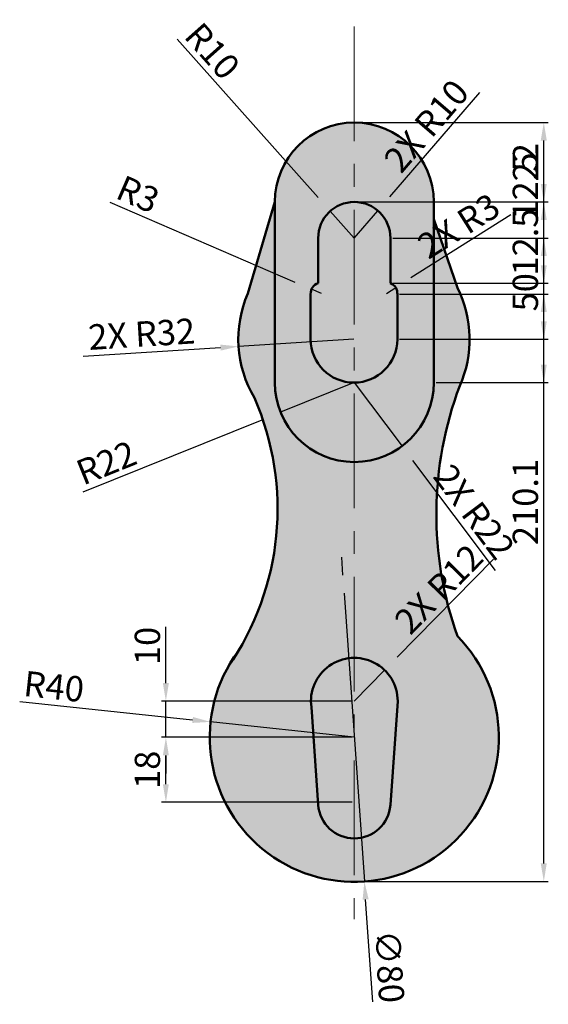
# Model space of a CAD drawing. Units: millimetres. Extents: x 3154 to 3300, y 2281 to 2553.
import ezdxf

# ---------------------------------------------------------------- set-up
doc = ezdxf.new("R2010")
doc.units = ezdxf.units.MM
doc.linetypes.add('CENTER', pattern=[50.8, 31.75, -6.35, 6.35, -6.35])
for name, color, linetype, lineweight in [('M-CNTR', 6, 'CENTER', 18), ('M-CONS', 8, 'Continuous', 13), ('M-DIMS', 2, 'Continuous', 25), ('M-HATC', 252, 'Continuous', 18), ('M-OUTL', 7, 'Continuous', 50)]:
    doc.layers.add(name, color=color, linetype=linetype, lineweight=lineweight)
doc.styles.get("Standard").update_dxf_attribs({"font": 'arial.ttf'})
doc.dimstyles.new('ISO-25', dxfattribs={"dimtxt": 7, "dimasz": 5, "dimexe": 1.25, "dimexo": 0.625, "dimtad": 1, "dimtxsty": 'Standard', "dimcen": 2.5, "dimadec": 0, "dimazin": 0, "dimtfac": 1, "dimtmove": 0, "dimatfit": 3, "dimfxl": 1, "dimarcsym": 0})

# ---------------------------------------------------------------- blocks, each defined once
blk = doc.blocks.new('*D1')
at = {"layer": 'Defpoints', "color": 0, "transparency": 16777216}
for p in [(3239.75, 2500.3), (3246.4, 2492.83)]:
    blk.add_point(p, dxfattribs=at)
at = {"layer": 'M-DIMS', "color": 0, "lineweight": -2, "transparency": 16777216}
for p, q in [((3197.36, 2547.92), (3236.43, 2504.03)), ((3246.4, 2492.83), (3239.75, 2500.3))]:
    blk.add_line(p, q, dxfattribs=at)
at = {"layer": 'M-DIMS', "color": 0, "transparency": 16777216}
blk.add_solid([(3237.05, 2504.59), (3235.8, 2503.48), (3239.75, 2500.3)], dxfattribs=at)
at = {"layer": 'M-DIMS', "color": 0, "transparency": 16777216, "insert": (3206.46, 2544.01), "char_height": 7, "attachment_point": 5, "rotation": 311.6742}
blk.add_mtext('R10', dxfattribs=at)
blk = doc.blocks.new('*D2')
at = {"layer": 'Defpoints', "color": 0, "transparency": 16777216}
for p in [(3246.4, 2452.83), (3225.99, 2444.61)]:
    blk.add_point(p, dxfattribs=at)
at = {"layer": 'M-DIMS', "color": 0, "lineweight": -2, "transparency": 16777216}
for p, q in [((3246.4, 2452.83), (3225.99, 2444.61)), ((3171.35, 2422.6), (3221.35, 2442.74))]:
    blk.add_line(p, q, dxfattribs=at)
at = {"layer": 'M-DIMS', "color": 0, "transparency": 16777216}
blk.add_solid([(3221.04, 2443.52), (3221.67, 2441.97), (3225.99, 2444.61)], dxfattribs=at)
at = {"layer": 'M-DIMS', "color": 0, "transparency": 16777216, "insert": (3178.11, 2429.79), "char_height": 7, "attachment_point": 5, "rotation": 21.936}
blk.add_mtext('R22', dxfattribs=at)
blk = doc.blocks.new('*D3')
at = {"layer": 'Defpoints', "color": 0, "transparency": 16777216}
for p in [(3234.55, 2478.66), (3237.3, 2477.47)]:
    blk.add_point(p, dxfattribs=at)
at = {"layer": 'M-DIMS', "color": 0, "lineweight": -2, "transparency": 16777216}
for p, q in [((3178.78, 2502.78), (3229.96, 2480.64)), ((3237.3, 2477.47), (3234.55, 2478.66))]:
    blk.add_line(p, q, dxfattribs=at)
at = {"layer": 'M-DIMS', "color": 0, "transparency": 16777216}
blk.add_solid([(3230.29, 2481.41), (3229.63, 2479.88), (3234.55, 2478.66)], dxfattribs=at)
at = {"layer": 'M-DIMS', "color": 0, "transparency": 16777216, "insert": (3186.2, 2504.15), "char_height": 7, "attachment_point": 5, "rotation": 336.611}
blk.add_mtext('R3', dxfattribs=at)
blk = doc.blocks.new('*D4')
at = {"layer": 'Defpoints', "color": 0, "transparency": 16777216}
for p in [(3206.63, 2358.9), (3246.4, 2354.63)]:
    blk.add_point(p, dxfattribs=at)
at = {"layer": 'M-DIMS', "color": 0, "lineweight": -2, "transparency": 16777216}
for p, q in [((3153.82, 2364.58), (3201.66, 2359.44)), ((3246.4, 2354.63), (3206.63, 2358.9))]:
    blk.add_line(p, q, dxfattribs=at)
at = {"layer": 'M-DIMS', "color": 0, "transparency": 16777216}
blk.add_solid([(3201.75, 2360.26), (3201.57, 2358.61), (3206.63, 2358.9)], dxfattribs=at)
at = {"layer": 'M-DIMS', "color": 0, "transparency": 16777216, "insert": (3163.19, 2367.8), "char_height": 7, "attachment_point": 5, "rotation": 353.8634}
blk.add_mtext('R40', dxfattribs=at)
blk = doc.blocks.new('*D5')
at = {"layer": 'Defpoints', "color": 0, "transparency": 16777216}
for p in [(3246.4, 2524.83), (3298.83, 2524.83), (3249.19, 2314.72)]:
    blk.add_point(p, dxfattribs=at)
at = {"layer": 'M-DIMS', "color": 0, "lineweight": -2, "transparency": 16777216}
for p, q in [((3247.02, 2524.83), (3300.08, 2524.83)), ((3298.83, 2319.72), (3298.83, 2519.83)), ((3249.81, 2314.72), (3300.08, 2314.72))]:
    blk.add_line(p, q, dxfattribs=at)
at = {"layer": 'M-DIMS', "color": 0, "transparency": 16777216}
for points in [[(3297.99, 2519.83), (3299.66, 2519.83), (3298.83, 2524.83)], [(3297.99, 2319.72), (3299.66, 2319.72), (3298.83, 2314.72)]]:
    blk.add_solid(points, dxfattribs=at)
at = {"layer": 'M-DIMS', "color": 0, "transparency": 16777216, "insert": (3294.63, 2419.78), "char_height": 7, "attachment_point": 5, "rotation": 90}
blk.add_mtext('210.1', dxfattribs=at)
blk = doc.blocks.new('*D6')
at = {"layer": 'Defpoints', "color": 0, "transparency": 16777216}
for p in [(3268.4, 2502.83), (3298.83, 2502.83), (3268.4, 2452.83)]:
    blk.add_point(p, dxfattribs=at)
at = {"layer": 'M-DIMS', "color": 0, "lineweight": -2, "transparency": 16777216}
for p, q in [((3269.02, 2502.83), (3300.08, 2502.83)), ((3298.83, 2457.83), (3298.83, 2497.83)), ((3269.02, 2452.83), (3300.08, 2452.83))]:
    blk.add_line(p, q, dxfattribs=at)
at = {"layer": 'M-DIMS', "color": 0, "transparency": 16777216}
for points in [[(3297.99, 2497.83), (3299.66, 2497.83), (3298.83, 2502.83)], [(3297.99, 2457.83), (3299.66, 2457.83), (3298.83, 2452.83)]]:
    blk.add_solid(points, dxfattribs=at)
at = {"layer": 'M-DIMS', "color": 0, "transparency": 16777216, "insert": (3294.63, 2477.83), "char_height": 7, "attachment_point": 5, "rotation": 90}
blk.add_mtext('50', dxfattribs=at)
blk = doc.blocks.new('*D7')
at = {"layer": 'Defpoints', "color": 0, "transparency": 16777216}
for p in [(3258.3, 2477.33), (3298.83, 2477.33), (3258.31, 2464.83)]:
    blk.add_point(p, dxfattribs=at)
at = {"layer": 'M-DIMS', "color": 0, "lineweight": -2, "transparency": 16777216}
for p, q in [((3298.83, 2477.33), (3298.83, 2501.16)), ((3258.92, 2477.33), (3300.08, 2477.33)), ((3298.83, 2469.83), (3298.83, 2472.33)), ((3258.93, 2464.83), (3300.08, 2464.83))]:
    blk.add_line(p, q, dxfattribs=at)
at = {"layer": 'M-DIMS', "color": 0, "transparency": 16777216}
for points in [[(3297.99, 2472.33), (3299.66, 2472.33), (3298.83, 2477.33)], [(3297.99, 2469.83), (3299.66, 2469.83), (3298.83, 2464.83)]]:
    blk.add_solid(points, dxfattribs=at)
at = {"layer": 'M-DIMS', "color": 0, "transparency": 16777216, "insert": (3294.63, 2491.74), "char_height": 7, "attachment_point": 5, "rotation": 90}
blk.add_mtext('12.5', dxfattribs=at)
blk = doc.blocks.new('*D8')
at = {"layer": 'Defpoints', "color": 0, "transparency": 16777216}
for p in [(3256.4, 2492.83), (3298.83, 2492.83), (3256.4, 2480.33)]:
    blk.add_point(p, dxfattribs=at)
at = {"layer": 'M-DIMS', "color": 0, "lineweight": -2, "transparency": 16777216}
for p, q in [((3298.83, 2492.83), (3298.83, 2516.66)), ((3257.02, 2492.83), (3300.08, 2492.83)), ((3298.83, 2485.33), (3298.83, 2487.83)), ((3257.02, 2480.33), (3300.08, 2480.33))]:
    blk.add_line(p, q, dxfattribs=at)
at = {"layer": 'M-DIMS', "color": 0, "transparency": 16777216}
for points in [[(3297.99, 2487.83), (3299.66, 2487.83), (3298.83, 2492.83)], [(3297.99, 2485.33), (3299.66, 2485.33), (3298.83, 2480.33)]]:
    blk.add_solid(points, dxfattribs=at)
at = {"layer": 'M-DIMS', "color": 0, "transparency": 16777216, "insert": (3294.63, 2507.24), "char_height": 7, "attachment_point": 5, "rotation": 90}
blk.add_mtext('12.5', dxfattribs=at)
blk = doc.blocks.new('*D9')
at = {"layer": 'Defpoints', "color": 0, "transparency": 16777216}
for p in [(3246.4, 2524.83), (3298.83, 2524.83), (3246.4, 2502.83)]:
    blk.add_point(p, dxfattribs=at)
at = {"layer": 'M-DIMS', "color": 0, "lineweight": -2, "transparency": 16777216}
for p, q in [((3247.02, 2524.83), (3300.08, 2524.83)), ((3298.83, 2507.83), (3298.83, 2519.83)), ((3247.02, 2502.83), (3300.08, 2502.83))]:
    blk.add_line(p, q, dxfattribs=at)
at = {"layer": 'M-DIMS', "color": 0, "transparency": 16777216}
for points in [[(3297.99, 2519.83), (3299.66, 2519.83), (3298.83, 2524.83)], [(3297.99, 2507.83), (3299.66, 2507.83), (3298.83, 2502.83)]]:
    blk.add_solid(points, dxfattribs=at)
at = {"layer": 'M-DIMS', "color": 0, "transparency": 16777216, "insert": (3294.69, 2513.83), "char_height": 7, "attachment_point": 5, "rotation": 90}
blk.add_mtext('22', dxfattribs=at)
blk = doc.blocks.new('*D10')
at = {"layer": 'Defpoints', "color": 0, "transparency": 16777216}
for p in [(3194.26, 2364.63), (3246.4, 2364.63), (3246.4, 2354.63)]:
    blk.add_point(p, dxfattribs=at)
at = {"layer": 'M-DIMS', "color": 0, "lineweight": -2, "transparency": 16777216}
for p, q in [((3194.26, 2369.63), (3194.26, 2385.22)), ((3245.77, 2364.63), (3193.01, 2364.63)), ((3194.26, 2354.63), (3194.26, 2364.63)), ((3245.77, 2354.63), (3193.01, 2354.63)), ((3194.26, 2349.63), (3194.26, 2344.63))]:
    blk.add_line(p, q, dxfattribs=at)
at = {"layer": 'M-DIMS', "color": 0, "transparency": 16777216}
for points in [[(3193.43, 2369.63), (3195.09, 2369.63), (3194.26, 2364.63)], [(3193.43, 2349.63), (3195.09, 2349.63), (3194.26, 2354.63)]]:
    blk.add_solid(points, dxfattribs=at)
at = {"layer": 'M-DIMS', "color": 0, "transparency": 16777216, "insert": (3190.06, 2379.92), "char_height": 7, "attachment_point": 5, "rotation": 90}
blk.add_mtext('10', dxfattribs=at)
blk = doc.blocks.new('*D11')
at = {"layer": 'Defpoints', "color": 0, "transparency": 16777216}
for p in [(3194.26, 2354.63), (3246.4, 2354.63), (3246.4, 2336.63)]:
    blk.add_point(p, dxfattribs=at)
at = {"layer": 'M-DIMS', "color": 0, "lineweight": -2, "transparency": 16777216}
for p, q in [((3245.77, 2354.63), (3193.01, 2354.63)), ((3194.26, 2341.63), (3194.26, 2349.63)), ((3245.77, 2336.63), (3193.01, 2336.63))]:
    blk.add_line(p, q, dxfattribs=at)
at = {"layer": 'M-DIMS', "color": 0, "transparency": 16777216}
for points in [[(3193.43, 2349.63), (3195.09, 2349.63), (3194.26, 2354.63)], [(3193.43, 2341.63), (3195.09, 2341.63), (3194.26, 2336.63)]]:
    blk.add_solid(points, dxfattribs=at)
at = {"layer": 'M-DIMS', "color": 0, "transparency": 16777216, "insert": (3190.06, 2345.63), "char_height": 7, "attachment_point": 5, "rotation": 90}
blk.add_mtext('18', dxfattribs=at)
blk = doc.blocks.new('*D12')
at = {"layer": 'Defpoints', "color": 0, "transparency": 16777216}
for p in [(3243.61, 2394.53), (3249.19, 2314.72)]:
    blk.add_point(p, dxfattribs=at)
at = {"layer": 'M-DIMS', "color": 0, "lineweight": -2, "transparency": 16777216}
for p, q in [((3243.26, 2399.52), (3242.91, 2404.5)), ((3243.61, 2394.53), (3249.19, 2314.72)), ((3251.52, 2281.37), (3249.54, 2309.74))]:
    blk.add_line(p, q, dxfattribs=at)
at = {"layer": 'M-DIMS', "color": 0, "transparency": 16777216}
for points in [[(3244.09, 2399.57), (3242.43, 2399.46), (3243.61, 2394.53)], [(3250.37, 2309.79), (3248.7, 2309.68), (3249.19, 2314.72)]]:
    blk.add_solid(points, dxfattribs=at)
at = {"layer": 'M-DIMS', "color": 0, "transparency": 16777216, "insert": (3255.24, 2291.09), "char_height": 7, "attachment_point": 5, "rotation": 273.9964}
blk.add_mtext('∅80', dxfattribs=at)
blk = doc.blocks.new('*D13')
at = {"layer": 'Defpoints', "color": 0, "transparency": 16777216}
for p in [(3246.4, 2452.83), (3259.61, 2435.24)]:
    blk.add_point(p, dxfattribs=at)
at = {"layer": 'M-DIMS', "color": 0, "lineweight": -2, "transparency": 16777216}
for p, q in [((3246.4, 2452.83), (3259.61, 2435.24)), ((3285.47, 2400.8), (3262.61, 2431.24))]:
    blk.add_line(p, q, dxfattribs=at)
at = {"layer": 'M-DIMS', "color": 0, "transparency": 16777216}
blk.add_solid([(3263.28, 2431.74), (3261.95, 2430.74), (3259.61, 2435.24)], dxfattribs=at)
at = {"layer": 'M-DIMS', "color": 0, "transparency": 16777216, "insert": (3278.85, 2416.51), "char_height": 7, "attachment_point": 5, "rotation": 306.9035}
blk.add_mtext('2X R22', dxfattribs=at)
blk = doc.blocks.new('*D14')
at = {"layer": 'Defpoints', "color": 0, "transparency": 16777216}
for p in [(3246.31, 2464.83), (3214.37, 2462.83)]:
    blk.add_point(p, dxfattribs=at)
at = {"layer": 'M-DIMS', "color": 0, "lineweight": -2, "transparency": 16777216}
for p, q in [((3246.31, 2464.83), (3214.37, 2462.83)), ((3171.39, 2460.14), (3209.38, 2462.52))]:
    blk.add_line(p, q, dxfattribs=at)
at = {"layer": 'M-DIMS', "color": 0, "transparency": 16777216}
blk.add_solid([(3209.33, 2463.35), (3209.43, 2461.68), (3214.37, 2462.83)], dxfattribs=at)
at = {"layer": 'M-DIMS', "color": 0, "transparency": 16777216, "insert": (3187.63, 2465.36), "char_height": 7, "attachment_point": 5, "rotation": 3.5837}
blk.add_mtext('2X R32', dxfattribs=at)
blk = doc.blocks.new('*D15')
at = {"layer": 'Defpoints', "color": 0, "transparency": 16777216}
for p in [(3257.85, 2479.13), (3255.32, 2477.53)]:
    blk.add_point(p, dxfattribs=at)
at = {"layer": 'M-DIMS', "color": 0, "lineweight": -2, "transparency": 16777216}
for p, q in [((3289.73, 2499.26), (3262.08, 2481.8)), ((3255.32, 2477.53), (3257.85, 2479.13))]:
    blk.add_line(p, q, dxfattribs=at)
at = {"layer": 'M-DIMS', "color": 0, "transparency": 16777216}
blk.add_solid([(3261.64, 2482.51), (3262.53, 2481.1), (3257.85, 2479.13)], dxfattribs=at)
at = {"layer": 'M-DIMS', "color": 0, "transparency": 16777216, "insert": (3275.77, 2495.42), "char_height": 7, "attachment_point": 5, "rotation": 32.2722}
blk.add_mtext('2X R3', dxfattribs=at)
blk = doc.blocks.new('*D16')
at = {"layer": 'Defpoints', "color": 0, "transparency": 16777216}
for p in [(3252.91, 2500.42), (3246.4, 2492.83)]:
    blk.add_point(p, dxfattribs=at)
at = {"layer": 'M-DIMS', "color": 0, "lineweight": -2, "transparency": 16777216}
for p, q in [((3281, 2533.13), (3256.17, 2504.21)), ((3246.4, 2492.83), (3252.91, 2500.42))]:
    blk.add_line(p, q, dxfattribs=at)
at = {"layer": 'M-DIMS', "color": 0, "transparency": 16777216}
blk.add_solid([(3255.54, 2504.75), (3256.8, 2503.67), (3252.91, 2500.42)], dxfattribs=at)
at = {"layer": 'M-DIMS', "color": 0, "transparency": 16777216, "insert": (3267.03, 2523.3), "char_height": 7, "attachment_point": 5, "rotation": 49.3492}
blk.add_mtext('2X R10', dxfattribs=at)
blk = doc.blocks.new('*D17')
at = {"layer": 'Defpoints', "color": 0, "transparency": 16777216}
for p in [(3254.8, 2373.2), (3246.4, 2364.63)]:
    blk.add_point(p, dxfattribs=at)
at = {"layer": 'M-DIMS', "color": 0, "lineweight": -2, "transparency": 16777216}
for p, q in [((3284.94, 2403.96), (3258.3, 2376.77)), ((3246.4, 2364.63), (3254.8, 2373.2))]:
    blk.add_line(p, q, dxfattribs=at)
at = {"layer": 'M-DIMS', "color": 0, "transparency": 16777216}
blk.add_solid([(3257.7, 2377.35), (3258.89, 2376.19), (3254.8, 2373.2)], dxfattribs=at)
at = {"layer": 'M-DIMS', "color": 0, "transparency": 16777216, "insert": (3270.41, 2395.05), "char_height": 7, "attachment_point": 5, "rotation": 45.5856}
blk.add_mtext('2X R12', dxfattribs=at)

msp = doc.modelspace()

# ---------------------------------------------------------------- hatches: boundary and pattern name
at = {"layer": 'M-HATC'}
h = msp.add_hatch(color=256, dxfattribs=at)
h.set_gradient(color1=(0, 0, 255), tint=1)
h.paths.add_polyline_path([(3246.399, 2502.829), (3246.399, 2524.829, 0.4142136), (3224.399, 2502.829), (3224.399, 2452.83, 0.4142136), (3246.399, 2430.83), (3246.399, 2452.83, -0.4164412), (3234.308, 2464.829), (3234.308, 2477.329, -0.3399266), (3236.399, 2480.329), (3236.399, 2492.829, -0.4142136)])
h = msp.add_hatch(color=256, dxfattribs=at)
h.set_gradient(color1=(255, 255, 255), color2=(0, 0, 255), tint=1)
h.paths.add_polyline_path([(3246.399, 2502.829, -0.4142136), (3256.399, 2492.829), (3256.399, 2480.329, -0.3304879), (3258.308, 2477.306), (3258.308, 2464.829, -0.4119894), (3246.399, 2452.83), (3246.399, 2430.83, 0.4142136), (3268.399, 2452.83), (3268.399, 2502.829, 0.4142136), (3246.399, 2524.829)])
h = msp.add_hatch(color=256, dxfattribs=at)
h.set_gradient(color1=(255, 0, 255), tint=1)
h.paths.add_polyline_path([(3211.479, 2374.133, 0.5726411), (3246.399, 2314.626), (3246.399, 2326.626, -0.393734), (3236.424, 2335.922), (3234.518, 2362.941, -0.4560954), (3246.399, 2376.626), (3246.399, 2430.83, -0.4142136), (3224.399, 2452.83), (3224.399, 2502.829), (3216.929, 2477.513, 0.2394804), (3218.741, 2448.579, -0.2603526)])
h = msp.add_hatch(color=256, dxfattribs=at)
h.set_gradient(color1=(255, 0, 0), color2=(241, 235, 31), tint=1, name='CYLINDER')
h.paths.add_polyline_path([(3236.399, 2492.829), (3236.399, 2480.329, 0.3399266), (3234.308, 2477.329), (3234.308, 2464.829, 0.4164412), (3246.399, 2452.83), (3246.399, 2502.829, 0.4142136)])
h.paths.add_polyline_path([(3246.399, 2452.83, 0.4119894), (3258.308, 2464.829), (3258.308, 2477.306, 0.3304879), (3256.399, 2480.329), (3256.399, 2492.829, 0.4142136), (3246.399, 2502.829)])
h = msp.add_hatch(color=256, dxfattribs=at)
h.set_gradient(color1=(255, 0, 255), tint=1)
h.paths.add_polyline_path([(3275.574, 2451.887, 0.223084), (3274.959, 2479.081), (3268.399, 2498.041), (3268.399, 2452.83, -0.4142136), (3246.399, 2430.83), (3246.399, 2376.626, -0.4142136), (3258.399, 2364.626), (3256.374, 2335.922, -0.393734), (3246.399, 2326.626), (3246.399, 2314.626, 0.6650433), (3274.928, 2382.663, -0.1775388)])
h = msp.add_hatch(color=256, dxfattribs=at)
h.set_gradient(color1=(255, 0, 0), color2=(241, 235, 31), tint=1, name='CYLINDER')
h.paths.add_polyline_path([(3246.399, 2376.626, 0.4560954), (3234.518, 2362.941), (3236.424, 2335.922, 0.393734), (3246.399, 2326.626)])
h.paths.add_polyline_path([(3258.399, 2364.626, 0.4142136), (3246.399, 2376.626), (3246.399, 2326.626, 0.393734), (3256.374, 2335.922)])

# ---------------------------------------------------------------- linework, layer by layer
at = {"layer": 'M-CNTR'}
msp.add_line((3246.399, 2551.442), (3246.399, 2304.318), dxfattribs=at)
at = {"layer": 'M-CONS'}
for centre, radius, start, end in [((3246.399, 2502.829), 22, 269.89821, 270), ((3246.399, 2492.829), 10, 269.81339, 270), ((3246.308, 2464.829), 12, 89.56457, 89.81339), ((3246.399, 2452.83), 22, 90, 90.15268)]:
    msp.add_arc(centre, radius, start, end, dxfattribs=at)
at = {"layer": 'M-OUTL'}
for p, q in [((3216.929, 2477.513), (3224.399, 2502.829)), ((3224.399, 2452.83), (3224.399, 2502.829)), ((3268.399, 2452.83), (3268.399, 2502.829)), ((3274.959, 2479.081), (3268.399, 2498.041)), ((3236.399, 2492.829), (3236.399, 2480.329)), ((3256.399, 2492.829), (3256.399, 2480.329)), ((3256.403, 2480.329), (3256.399, 2480.329)), ((3234.281, 2477.329), (3234.308, 2477.329)), ((3234.308, 2464.829), (3234.308, 2477.329)), ((3258.295, 2477.329), (3258.308, 2477.329)), ((3258.308, 2464.829), (3258.308, 2477.329)), ((3258.399, 2364.626), (3256.374, 2335.922)), ((3234.518, 2362.941), (3236.424, 2335.922))]:
    msp.add_line(p, q, dxfattribs=at)
for centre, radius, start, end in [((3246.399, 2502.829), 22, 0, 180), ((3246.399, 2492.829), 10, 0, 180), ((3237.305, 2477.469), 3, 107.56893, 182.66597), ((3255.317, 2477.531), 3, 355.69178, 68.84416), ((3246.308, 2464.829), 32, 336.14439, 26.44781), ((3246.308, 2464.829), 32, 156.64915, 210.51947), ((3246.308, 2464.829), 12, 180, 0), ((3246.399, 2452.83), 22, 180, 0), ((3369.656, 2416.394), 100.554, 159.33053, 199.59984), ((3148.471, 2417.857), 76.693, 325.24159, 23.61415), ((3246.399, 2354.626), 40, 143.48907, 44.50251), ((3246.399, 2364.626), 12, 0, 188.07005), ((3246.399, 2336.626), 10, 184.03502, 355.96498)]:
    msp.add_arc(centre, radius, start, end, dxfattribs=at)

# ---------------------------------------------------------------- dimensions: what is measured, and where the dimension line sits
at = {"layer": 'M-DIMS'}
for center, mpoint, picture, middle in [((3246.399, 2492.829), (3239.75, 2500.298), '*D1', (3203.325, 2541.218)), ((3237.305, 2477.469), (3234.551, 2478.66), '*D3', (3184.536, 2500.292)), ((3246.399, 2452.83), (3225.992, 2444.611), '*D2', (3179.651, 2425.948)), ((3246.399, 2354.626), (3206.628, 2358.902), '*D4', (3162.742, 2363.62))]:
    dim = msp.add_radius_dim(center=center, mpoint=mpoint, dimstyle='ISO-25', override={"dimclrd": 0, "dimclre": 0, "dimclrt": 0}, dxfattribs=at)
    dim.commit()
    dim.dimension.update_dxf_attribs({"geometry": picture, "text_midpoint": middle, "dimtype": 164})
for center, mpoint, picture, middle in [((3246.399, 2492.829), (3252.914, 2500.416), '*D16', (3267.028, 2523.3)), ((3255.317, 2477.531), (3257.853, 2479.133), '*D15', (3275.775, 2495.419)), ((3246.308, 2464.829), (3214.371, 2462.829), '*D14', (3187.627, 2465.364)), ((3246.399, 2452.83), (3259.61, 2435.237), '*D13', (3278.853, 2416.508)), ((3246.399, 2364.626), (3254.797, 2373.197), '*D17', (3270.408, 2395.048))]:
    dim = msp.add_radius_dim(center=center, mpoint=mpoint, text='2X <>', dimstyle='ISO-25', override={"dimdec": 0, "dimlfac": 1, "dimrnd": 0, "dimzin": 0, "dimdsep": 46, "dimlunit": 2}, dxfattribs=at)
    dim.commit()
    dim.dimension.update_dxf_attribs({"geometry": picture, "text_midpoint": middle})
for base, p1, p2, override, picture, middle in [((3298.828, 2524.829), (3249.187, 2314.723), (3246.399, 2524.829), {"dimdec": 1, "dimlfac": 1, "dimrnd": 0, "dimzin": 0, "dimdsep": 46, "dimlunit": 2}, '*D5', (3294.629, 2419.776)), ((3298.828, 2524.829), (3246.399, 2502.829), (3246.399, 2524.829), {"dimdec": 0, "dimlfac": 1, "dimrnd": 0, "dimzin": 0, "dimdsep": 46, "dimlunit": 2}, '*D9', (3294.689, 2513.829)), ((3298.828, 2492.829), (3256.399, 2480.329), (3256.399, 2492.829), {"dimdec": 1, "dimlfac": 1, "dimrnd": 0, "dimzin": 0, "dimdsep": 46, "dimlunit": 2}, '*D8', (3294.629, 2507.242)), ((3298.828, 2502.829), (3268.399, 2452.83), (3268.399, 2502.829), {"dimdec": 0, "dimlfac": 1, "dimrnd": 0, "dimzin": 0, "dimdsep": 46, "dimlunit": 2}, '*D6', (3294.629, 2477.829)), ((3298.828, 2477.329), (3258.308, 2464.829), (3258.295, 2477.329), {"dimdec": 1, "dimlfac": 1, "dimrnd": 0, "dimzin": 0, "dimdsep": 46, "dimlunit": 2}, '*D7', (3294.629, 2491.742)), ((3194.262, 2364.626), (3246.399, 2354.626), (3246.399, 2364.626), {"dimdec": 0, "dimlfac": 1, "dimrnd": 0, "dimzin": 0, "dimdsep": 46, "dimlunit": 2}, '*D10', (3190.063, 2379.923)), ((3194.262, 2354.626), (3246.399, 2336.626), (3246.399, 2354.626), {"dimdec": 0, "dimlfac": 1, "dimrnd": 0, "dimzin": 0, "dimdsep": 46, "dimlunit": 2}, '*D11', (3190.063, 2345.626))]:
    dim = msp.add_linear_dim(base=base, p1=p1, p2=p2, angle=90, dimstyle='ISO-25', override=override, dxfattribs=at)
    dim.commit()
    dim.dimension.update_dxf_attribs({"geometry": picture, "text_midpoint": middle})
dim = msp.add_diameter_dim_2p(p1=(3243.611, 2394.528), p2=(3249.187, 2314.723), dimstyle='ISO-25', override={"dimdec": 0, "dimlfac": 1, "dimrnd": 0, "dimzin": 0, "dimdsep": 46, "dimlunit": 2}, dxfattribs=at)
dim.commit()
dim.dimension.update_dxf_attribs({"geometry": '*D12', "text_midpoint": (3250.86, 2290.781), "dimtype": 163})

doc.saveas('drawing.dxf')
